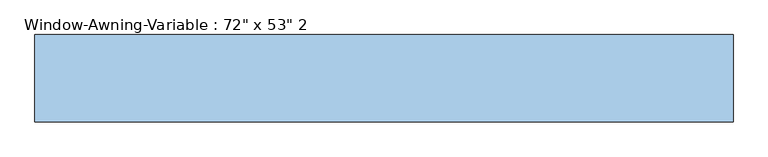
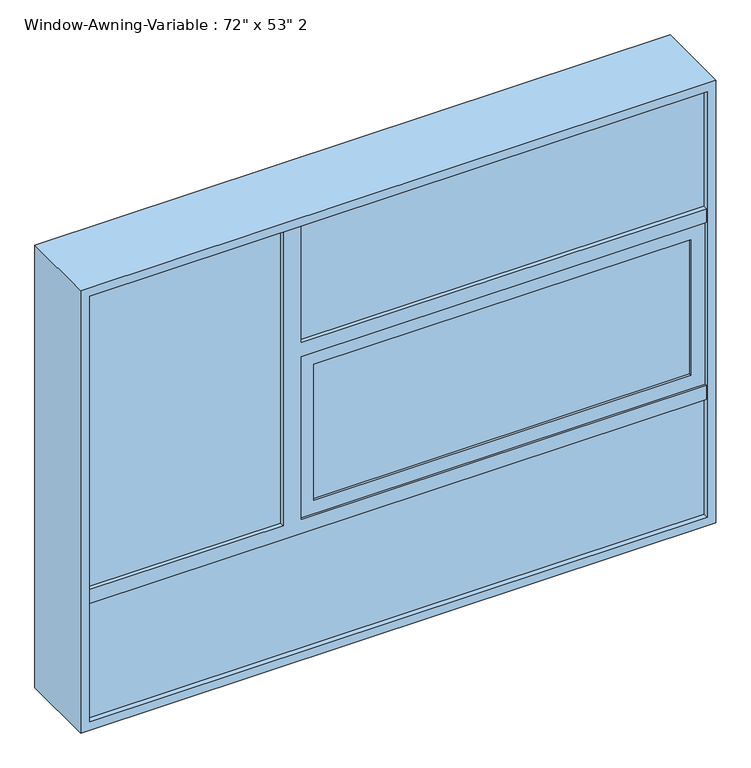
"""IFC4 building model written with IfcOpenShell, lengths in millimetres: window geometry."""

from ifc_helpers import new_model, si_unit, frame, origin, place, context, project, spatial, polyline, outline, extrude, faceted_brep, source, transform, mapped, element, save


def window_511101a2(model_context):
    return source(origin(), model_context, "Body", "SolidModel", [
        extrude(outline(polyline([(847.1296875, -98.425), (-237.5296875, -98.425), (-237.5296875, -92.075), (847.1296875, -92.075), (847.1296875, -98.425)])), frame((0.0, 0.0, 1381.0654688), z_axis=(0.0, 0.0, 1.0), x_axis=(1.0, 0.0, 0.0)), (0.0, 0.0, 1.0), 412.8690625),
        extrude(outline(polyline([(847.1296875, -85.725), (-237.5296875, -85.725), (-237.5296875, -79.375), (847.1296875, -79.375), (847.1296875, -85.725)])), frame((0.0, 0.0, 1381.0654688), z_axis=(0.0, 0.0, 1.0), x_axis=(1.0, 0.0, 0.0)), (0.0, 0.0, 1.0), 412.8690625),
        extrude(outline(polyline([(-330.2, -98.425), (-889.0, -98.425), (-889.0, -92.075), (-330.2, -92.075), (-330.2, -98.425)])), frame((0.0, 0.0, 1339.1951563), z_axis=(0.0, 0.0, 1.0), x_axis=(1.0, 0.0, 0.0)), (0.0, 0.0, 1.0), 896.0048438),
        extrude(outline(polyline([(-330.2, -85.725), (-889.0, -85.725), (-889.0, -79.375), (-330.2, -79.375), (-330.2, -85.725)])), frame((0.0, 0.0, 1339.1951563), z_axis=(0.0, 0.0, 1.0), x_axis=(1.0, 0.0, 0.0)), (0.0, 0.0, 1.0), 896.0048438),
        extrude(outline(polyline([(889.0, -85.725), (-279.4, -85.725), (-279.4, -79.375), (889.0, -79.375), (889.0, -85.725)])), frame((0.0, 0.0, 1877.6751563), z_axis=(0.0, 0.0, 1.0), x_axis=(1.0, 0.0, 0.0)), (0.0, 0.0, 1.0), 357.5248438),
        extrude(outline(polyline([(889.0, -98.425), (-279.4, -98.425), (-279.4, -92.075), (889.0, -92.075), (889.0, -98.425)])), frame((0.0, 0.0, 1877.6751563), z_axis=(0.0, 0.0, 1.0), x_axis=(1.0, 0.0, 0.0)), (0.0, 0.0, 1.0), 357.5248438),
        extrude(outline(polyline([(889.0, -98.425), (-889.0, -98.425), (-889.0, -92.075), (889.0, -92.075), (889.0, -98.425)])), frame((0.0, 0.0, 939.8), z_axis=(0.0, 0.0, 1.0), x_axis=(1.0, 0.0, 0.0)), (0.0, 0.0, 1.0), 357.5248438),
        extrude(outline(polyline([(889.0, -85.725), (-889.0, -85.725), (-889.0, -79.375), (889.0, -79.375), (889.0, -85.725)])), frame((0.0, 0.0, 939.8), z_axis=(0.0, 0.0, 1.0), x_axis=(1.0, 0.0, 0.0)), (0.0, 0.0, 1.0), 357.5248438),
        faceted_brep([(-889.0, -73.025, 2235.2), (-330.2, -73.025, 2235.2), (-330.2, -111.125, 2235.2), (-279.4, -111.125, 2235.2), (-279.4, -73.025, 2235.2), (889.0, -73.025, 2235.2), (889.0, -114.3, 2235.2), (-889.0, -114.3, 2235.2), (-878.8796875, -42.06875, 2225.0796875), (-330.2, -42.06875, 2225.0796875), (-330.2, -73.025, 2225.0796875), (-878.8796875, -73.025, 2225.0796875), (878.8796875, -73.025, 2225.0796875), (-269.2796875, -73.025, 2225.0796875), (-269.2796875, -42.06875, 2225.0796875), (878.8796875, -42.06875, 2225.0796875), (-889.0, 114.3, 2235.2), (889.0, 114.3, 2235.2), (889.0, -42.06875, 2235.2), (-889.0, -42.06875, 2235.2), (-914.4, -114.3, 2260.6), (914.4, -114.3, 2260.6), (914.4, 114.3, 2260.6), (-914.4, 114.3, 2260.6), (889.0, -73.025, 1877.6751563), (889.0, -111.125, 1877.6751563), (889.0, -111.125, 1835.8048438), (889.0, -73.025, 1835.8048438), (889.0, -73.025, 1339.1951563), (889.0, -111.125, 1339.1951563), (889.0, -111.125, 1297.3248438), (889.0, -73.025, 1297.3248438), (889.0, -73.025, 939.8), (889.0, -114.3, 939.8), (878.8796875, -42.06875, 1877.6751563), (878.8796875, -73.025, 1877.6751563), (878.8796875, -73.025, 949.9203125), (878.8796875, -73.025, 1297.3248438), (878.8796875, -42.06875, 1297.3248438), (878.8796875, -42.06875, 949.9203125), (878.8796875, -73.025, 1339.1951563), (878.8796875, -73.025, 1835.8048438), (878.8796875, -42.06875, 1835.8048438), (878.8796875, -42.06875, 1339.1951563), (889.0, 114.3, 939.8), (889.0, -42.06875, 939.8), (914.4, -114.3, 914.4), (914.4, 114.3, 914.4), (-889.0, -73.025, 939.8), (-889.0, -114.3, 939.8), (-878.8796875, -42.06875, 949.9203125), (-878.8796875, -73.025, 949.9203125), (-889.0, 114.3, 939.8), (-889.0, -42.06875, 939.8), (-914.4, -114.3, 914.4), (-914.4, 114.3, 914.4), (-889.0, -73.025, 1297.3248438), (-889.0, -111.125, 1297.3248438), (-889.0, -111.125, 1339.1951563), (-889.0, -73.025, 1339.1951563), (-878.8796875, -73.025, 1297.3248438), (-279.4, -73.025, 1877.6751563), (-269.2796875, -73.025, 1877.6751563), (-878.8796875, -73.025, 1339.1951563), (-269.2796875, -73.025, 1339.1951563), (-269.2796875, -73.025, 1835.8048438), (-279.4, -73.025, 1835.8048438), (-279.4, -73.025, 1339.1951563), (-878.8796875, -42.06875, 1339.1951563), (-878.8796875, -42.06875, 1297.3248438), (-330.2, -42.06875, 1339.1951563), (-269.2796875, -42.06875, 1877.6751563), (-269.2796875, -42.06875, 1339.1951563), (-269.2796875, -42.06875, 1835.8048438), (-279.4, -111.125, 1339.1951563), (-279.4, -111.125, 1835.8048438), (-279.4, -111.125, 1877.6751563), (-330.2, -111.125, 1339.1951563)], [[[0, 1, 2, 3, 4, 5, 6, 7]], [[8, 9, 10, 11]], [[12, 13, 14, 15]], [[16, 17, 18, 19]], [[20, 21, 22, 23]], [[5, 24, 25, 26, 27, 28, 29, 30, 31, 32, 33, 6]], [[15, 34, 35, 12]], [[36, 37, 38, 39]], [[40, 41, 42, 43]], [[17, 44, 45, 18]], [[21, 46, 47, 22]], [[32, 48, 49, 33]], [[39, 50, 51, 36]], [[44, 52, 53, 45]], [[46, 54, 55, 47]], [[7, 49, 48, 56, 57, 58, 59, 0]], [[32, 31, 37, 36, 51, 60, 56, 48]], [[28, 27, 41, 40]], [[12, 35, 24, 5, 4, 61, 62, 13]], [[59, 63, 11, 10, 1, 0]], [[64, 65, 66, 67]], [[11, 63, 68, 8]], [[50, 69, 60, 51]], [[53, 19, 18, 45], [39, 38, 69, 50], [68, 70, 9, 8], [14, 71, 34, 15], [72, 43, 42, 73]], [[19, 53, 52, 16]], [[22, 47, 55, 23], [16, 52, 44, 17]], [[23, 55, 54, 20]], [[20, 54, 46, 21], [6, 33, 49, 7]], [[57, 56, 60, 69, 38, 37, 31, 30]], [[30, 29, 74, 75, 26, 25, 76, 3, 2, 77, 58, 57]], [[28, 40, 43, 72, 64, 67, 74, 29]], [[58, 77, 70, 68, 63, 59]], [[2, 1, 10, 9, 70, 77]], [[13, 62, 71, 14]], [[72, 73, 65, 64]], [[67, 66, 75, 74]], [[3, 76, 61, 4]], [[75, 66, 65, 73, 42, 41, 27, 26]], [[25, 24, 35, 34, 71, 62, 61, 76]]]),
        extrude(outline(polyline([(1339.1951563, -279.4), (1339.1951563, 889.0), (1835.8048438, 889.0), (1835.8048438, -279.4), (1339.1951563, -279.4)]), holes=[polyline([(1381.0654688, -237.5296875), (1793.9345313, -237.5296875), (1793.9345313, 847.1296875), (1381.0654688, 847.1296875), (1381.0654688, -237.5296875)])]), frame((0.0, -104.775, 0.0), z_axis=(0.0, 1.0, 0.0), x_axis=(0.0, 0.0, 1.0)), (0.0, 0.0, 1.0), 31.75),
    ])


if __name__ == "__main__":
    model = new_model("IFC4")
    model_context = context("Model", 3, world=origin())
    ifc_project = project(units=[si_unit("LENGTHUNIT", "METRE", prefix="MILLI")], contexts=[model_context])
    site = spatial("IfcSite", under=ifc_project)
    building = spatial("IfcBuilding", under=site)
    placement = place(None, origin())
    window_shape = window_511101a2(model_context)
    element("IfcWindow", 1, ObjectType="Window-Awning-Variable : 72\" x 53\" 2", at=placement, inside=building, context=model_context, shape_type="MappedRepresentation", body=[
        mapped(window_shape, transform((0.0, 0.0, 0.0), x_axis=(1.0, 0.0, 0.0), y_axis=(0.0, 1.0, 0.0), z_axis=(0.0, 0.0, 1.0))),
    ])
    save(model, "model.ifc")

# Revit data of these elements
# Type "Window-Awning-Variable : 72\" x 53\" 2"
#   Type Mark = "21"
#   Fire Rating = "0.5h"
#   Assembly Code = "B2020100"
#   Analytic Construction = "Double glazing - domestic"
#   Window Inset [instance default] = 0' - 0 5/8"
#   Wall Thickness [instance default] = 0' - 6"
#   Visual Light Transmittance = 0.81
#   Transom Height Ratio = 0.3
#   Transom Height = 1' - 3.9"
#   Thermal Resistance (R) = 1.8146 (h·ft²·°F)/BTU
#   Solar Heat Gain Coefficient = 0.76
#   Rough Width = 6' - 0 1/2"
#   Rough Height = 4' - 5 1/2"
#   Opening Window Width = 4' - 0"
#   Opening Window Height = 1' - 9.2"
#   Heat Transfer Coefficient (U) = 0.5511 BTU/(h·ft²·°F)
#   Height = 4' - 5"
#   Frame Gap 3 [instance default] = 0' - 1 83/128"
#   Frame Gap 2 [instance default] = 0' - 0 5/8"
#   Frame Gap 1 = 0' - 1 51/128"
#   Fixed Window Width = 2' - 0"
#   Default Sill Height = 3' - 0"
#   Width = 6' - 0"
#   Frame Material = metal black
#   Glass Panel Material = Glass
#   Wall Closure = (empty or 0)
# Element 1 (IfcWindow, "Window-Awning-Variable : 72\" x 53\" 2")
#   Wall Thickness = 0' - 9"
#   Materials on its faces: "Glass", "metal black"
# Materials
#   "metal black": class "Generic", colour RGB 120 120 120, transparency 0, Cost = 0
#   "Glass": class "Glass", colour RGB 0 128 192, transparency 0.75, Description = "Soda Lime Glass", Cost = 0
